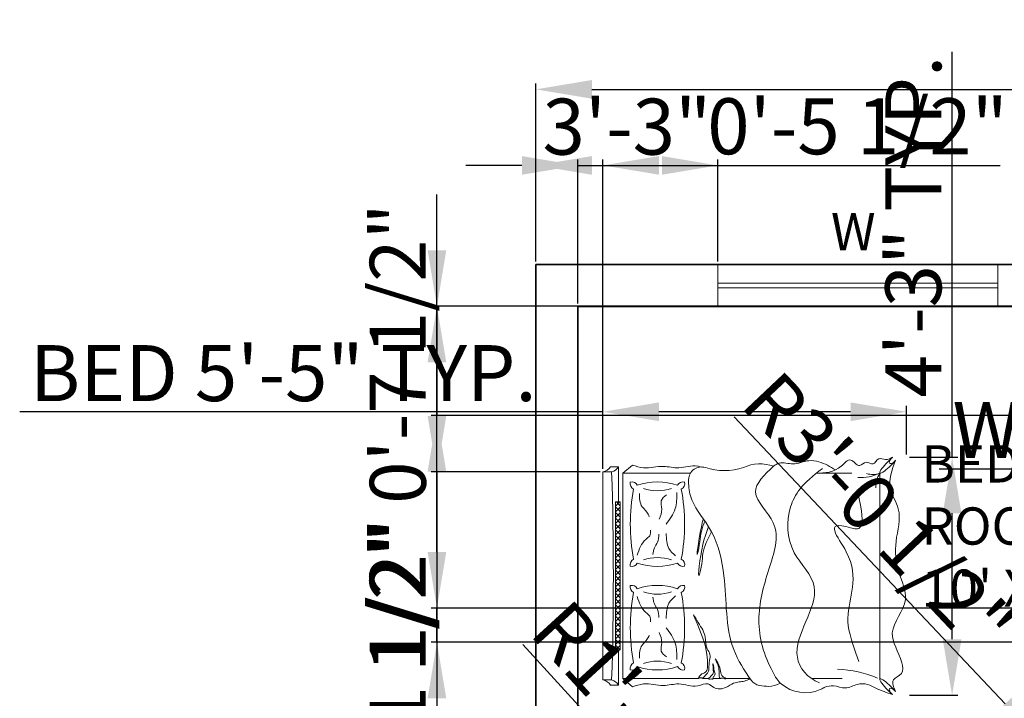
# Model space of a CAD drawing. Units: inches. Extents: x 2122 to 2726, y 1923 to 2370.
# Tile 3 of 6: x 2122 to 2333, y 2178 to 2324. Entities that reach past the tile are written whole.
import ezdxf

# ---------------------------------------------------------------- set-up
doc = ezdxf.new("R2010")
doc.units = ezdxf.units.IN
for name, color, linetype, lineweight in [('A-ANNO-DIMS', 2, 'Continuous', 18), ('A-ANNO-TEXT', 7, 'Continuous', 18), ('A-AREA-IDEN', 7, 'Continuous', 25), ('A-FURN', 8, 'Continuous', 18), ('A-GLAZ', 4, 'Continuous', 18), ('A-WALL', 7, 'Continuous', 35), ('www.cadblocksfree.com', 7, 'Continuous', 9)]:
    doc.layers.add(name, color=color, linetype=linetype, lineweight=lineweight)
doc.styles.get("Standard").update_dxf_attribs({"font": 'arial.ttf'})
doc.dimstyles.new('ISO-25', dxfattribs={"dimtxt": 12, "dimasz": 12, "dimexe": 1.25, "dimexo": 0.625, "dimtad": 1, "dimlunit": 3, "dimtxsty": 'Standard', "dimcen": 2.5, "dimadec": 0, "dimazin": 0, "dimtfac": 1, "dimtmove": 0, "dimatfit": 3, "dimfxl": 1, "dimarcsym": 0})

# ---------------------------------------------------------------- blocks, each defined once
blk = doc.blocks.new('bed')
at = {"layer": 'www.cadblocksfree.com', "ltscale": 0.2}
h = blk.add_hatch(dxfattribs=at)
h.set_pattern_fill('ANSI37,_O', color=256, scale=0.393701)
h.set_pattern_definition([(45, (2420.7222, -262.9689), (-0.8838835, 0.8838835), []), (135, (2420.7222, -262.9689), (-0.8838835, -0.8838835), [])])
h.paths.add_polyline_path([(3417.57, 1472.4), (3372.19, 1472.4), (3372.19, 1470.94), (3417.57, 1470.94)])
for p, q in [((3363, 1473.59), (3363, 1476.25)), ((3426.76, 1473.59), (3426.76, 1476.25)), ((3363.39, 1470.15), (3360.88, 1467.22)), ((3372.19, 1472.4), (3417.57, 1472.4)), ((3372.19, 1470.94), (3372.19, 1472.4)), ((3372.19, 1470.94), (3417.57, 1470.94)), ((3417.57, 1470.94), (3417.57, 1472.4)), ((3426.38, 1470.15), (3428.88, 1467.22)), ((3409.94, 1443.85), (3408.41, 1442.96)), ((3363.39, 1412.3), (3363.39, 1402.94)), ((3426.38, 1399.91), (3426.38, 1410.81)), ((3363.39, 1391.41), (3426.38, 1391.41))]:
    blk.add_line(p, q, dxfattribs=at)
for points in [[(3426.76, 1476.25), (3363, 1476.25)], [(3361.42, 1473.89), (3361.42, 1471.52), (3372.19, 1471.52)], [(3417.57, 1471.52), (3428.35, 1471.52), (3428.35, 1473.89)], [(3426.38, 1449.41), (3426.38, 1470.15), (3363.39, 1470.15), (3363.39, 1447.08)], [(3363.39, 1445.54), (3363.39, 1443.89)], [(3363.39, 1442.49), (3363.39, 1440.37)], [(3363.39, 1438.56), (3363.39, 1431.14)]]:
    blk.add_lwpolyline(points, dxfattribs=at)
for centre, radius, start, end in [((3359.33, 1477), 3.74, 303.8271, 348.4775), ((3430.43, 1477), 3.74, 191.5225, 236.1729), ((3359.84, 1474.37), 3.25, 298.9176, 345.9939), ((3394.88, 2431.36), 958.3, 268.09356, 271.90644), ((3429.92, 1474.37), 3.25, 194.0061, 241.0824), ((3367.9, 1467.4), 1.87, 165.5166, 244.2099), ((3366.56, 1466.05), 1.87, 25.7901, 104.4834), ((3379.01, 1409.19), 58.68, 79.4235, 100.5765), ((3391.47, 1466.05), 1.87, 75.5166, 154.2099), ((3390.12, 1467.4), 1.87, 295.7901, 14.4834), ((3399.64, 1467.4), 1.87, 165.5166, 244.2099), ((3398.3, 1466.05), 1.87, 25.7901, 104.4834), ((3410.75, 1409.19), 58.68, 79.4235, 100.5765), ((3423.21, 1466.05), 1.87, 75.5166, 154.2099), ((3421.86, 1467.4), 1.87, 295.7901, 14.4834), ((3385.29, 1459.55), 19.22, 161.2852, 198.7148), ((3355.42, 1459.55), 13.34, 341.1598, 18.8402), ((3402.61, 1459.55), 13.34, 161.1598, 198.8402), ((3372.74, 1459.55), 19.22, 341.2852, 18.7148), ((3417.03, 1459.55), 19.22, 161.2852, 198.7148), ((3387.15, 1459.55), 13.34, 341.1598, 18.8402), ((3434.35, 1459.55), 13.34, 161.1598, 198.8402), ((3404.48, 1459.55), 19.22, 341.2852, 18.7148), ((3367.9, 1451.7), 1.87, 115.7901, 194.4834), ((3366.56, 1453.04), 1.87, 255.5166, 334.2099), ((3379.01, 1509.91), 58.68, 259.4235, 280.5765), ((3391.47, 1453.04), 1.87, 205.7901, 284.4834), ((3390.12, 1451.7), 1.87, 345.5166, 64.2099), ((3399.64, 1451.7), 1.87, 115.7901, 194.4834), ((3398.3, 1453.04), 1.87, 255.5166, 334.2099), ((3410.75, 1509.91), 58.68, 259.4235, 280.5765), ((3423.21, 1453.04), 1.87, 205.7901, 284.4834), ((3421.86, 1451.7), 1.87, 345.5166, 64.2099), ((3424.34, 1446.05), 3.94, 342.0511, 87.9851), ((3445.78, 1439.1), 18.6, 162.0511, 198.5657), ((3365.21, 1427.6), 3.94, 125.4209, 169.6982), ((3416.57, 1428.08), 12.65, 341.0268, 23.7782), ((3370.55, 1414.19), 11.47, 139.4648, 203.3712), ((3367.28, 1412.87), 7.94, 204.0179, 212.619), ((3331.91, 1405.56), 34.38, 336.8495, 357.9003), ((3438.82, 1397.31), 13.77, 176.7525, 205.373), ((3432.14, 1393.64), 6.17, 162.6475, 201.1361), ((3422.11, 1384.8), 7.8, 58.0013, 91.6551)]:
    blk.add_arc(centre, radius, start, end, dxfattribs=at)
at = {"layer": 'www.cadblocksfree.com', "ltscale": 0.2, "extrusion": (0, 0, -1)}
for centre, major_axis, ratio, start_param, end_param in [((3360.34, 1388.37), (3.04, 3.04), 0.168252, 4.250342, 8.316029), ((3359.29, 1387.32), (1.05, 1.05), 0.453532, 4.422107, 8.144264)]:
    blk.add_ellipse(centre, major_axis=major_axis, ratio=ratio, start_param=start_param, end_param=end_param, dxfattribs=at)
at = {"layer": 'www.cadblocksfree.com', "ltscale": 0.2}
for centre, major_axis, ratio, start_param, end_param in [((3429.42, 1388.37), (-3.04, 3.04), 0.168252, 4.250342, 8.316029), ((3430.48, 1387.32), (-1.05, 1.05), 0.453532, 4.422107, 8.144264)]:
    blk.add_ellipse(centre, major_axis=major_axis, ratio=ratio, start_param=start_param, end_param=end_param, dxfattribs=at)
for points, knots in [([(3360.88, 1467.22), (3361.27, 1466.08), (3362.33, 1462.98), (3360.73, 1458.15), (3362.39, 1452.62), (3360.35, 1448.14), (3362.43, 1444.24), (3360.04, 1441.93), (3360.26, 1438.68), (3362.05, 1436.55), (3362.42, 1434.52), (3362.57, 1432.76), (3363.1, 1431.71), (3363.39, 1431.14)], [0, 0, 0, 0, 3.550403, 9.643115, 14.356056, 20.206026, 23.427697, 25.46537, 29.172767, 31.884544, 33.668442, 35.237641, 37.145618, 37.145618, 37.145618, 37.145618]), ([(3428.88, 1467.22), (3428.49, 1466.08), (3427.44, 1462.98), (3429.04, 1458.15), (3427.38, 1452.62), (3429.08, 1448.87), (3428.37, 1446.52), (3428.27, 1446.19)], [0, 0, 0, 0, 0.0901802, 0.2449351, 0.3646438, 0.5132331, 0.5378548, 0.5378548, 0.5378548, 0.5378548]), ([(3369.63, 1465.08), (3371.1, 1465.04), (3373.63, 1464.97), (3375.26, 1462.52), (3376.48, 1462.17), (3376.75, 1462.09)], [0, 0, 0, 0, 4.163459, 7.093919, 7.934624, 7.934624, 7.934624, 7.934624]), ([(3388.54, 1465.74), (3386.72, 1465.16), (3384.36, 1464.41), (3382.68, 1461.63), (3381.45, 1461.64), (3380.81, 1461.64)], [0, 0, 0, 0, 5.530688, 7.154877, 8.940839, 8.940839, 8.940839, 8.940839]), ([(3401.22, 1465.74), (3403.05, 1465.16), (3405.41, 1464.41), (3407.09, 1461.63), (3408.31, 1461.64), (3408.95, 1461.64)], [0, 0, 0, 0, 5.530688, 7.154877, 8.940839, 8.940839, 8.940839, 8.940839]), ([(3420.14, 1465.08), (3418.66, 1465.04), (3416.14, 1464.97), (3414.5, 1462.52), (3413.28, 1462.17), (3413.01, 1462.09)], [0, 0, 0, 0, 4.163459, 7.093919, 7.934624, 7.934624, 7.934624, 7.934624]), ([(3388.36, 1460.93), (3387.64, 1460.85), (3386.25, 1460.69), (3384.48, 1459.22), (3382.96, 1459.13), (3382.11, 1459.07)], [0, 0, 0, 0, 2.127543, 4.10272, 6.58647, 6.58647, 6.58647, 6.58647]), ([(3401.41, 1460.93), (3402.13, 1460.85), (3403.51, 1460.69), (3405.28, 1459.22), (3406.81, 1459.13), (3407.65, 1459.07)], [0, 0, 0, 0, 2.127543, 4.10272, 6.58647, 6.58647, 6.58647, 6.58647]), ([(3370.05, 1456.77), (3370.59, 1457.46), (3371.71, 1458.88), (3374.68, 1457.89), (3376.51, 1458.59), (3377.52, 1458.99)], [0, 0, 0, 0, 2.388143, 4.935423, 8.166198, 8.166198, 8.166198, 8.166198]), ([(3419.72, 1456.77), (3419.17, 1457.46), (3418.05, 1458.88), (3415.08, 1457.89), (3413.26, 1458.59), (3412.24, 1458.99)], [0, 0, 0, 0, 2.388143, 4.935423, 8.166198, 8.166198, 8.166198, 8.166198]), ([(3369.29, 1453.58), (3371, 1453.6), (3374.59, 1453.64), (3377.5, 1455.76), (3379.02, 1456.87)], [0, 0, 0, 0, 5.002087, 10.507046, 10.507046, 10.507046, 10.507046]), ([(3388.77, 1454), (3388.07, 1454.76), (3386.27, 1456.73), (3383.54, 1456.81), (3381.88, 1456.86)], [0, 0, 0, 0, 3.013696, 7.735839, 7.735839, 7.735839, 7.735839]), ([(3401, 1454), (3401.7, 1454.76), (3403.5, 1456.73), (3406.22, 1456.81), (3407.88, 1456.86)], [0, 0, 0, 0, 3.013696, 7.735839, 7.735839, 7.735839, 7.735839]), ([(3420.48, 1453.58), (3418.77, 1453.6), (3415.18, 1453.64), (3412.27, 1455.76), (3410.74, 1456.87)], [0, 0, 0, 0, 5.002087, 10.507046, 10.507046, 10.507046, 10.507046]), ([(3367.27, 1444.2), (3369.57, 1444.23), (3373.92, 1444.28), (3385.47, 1449.8), (3379.56, 1446.49), (3376.81, 1444.48), (3372.95, 1444.92), (3370.93, 1443.14), (3368.77, 1443.7), (3367.36, 1443.75), (3366.55, 1443.78)], [0, 0, 0, 0, 8.61026, 16.221274, 18.843057, 23.804898, 27.440828, 29.356102, 31.203478, 33.650687, 33.650687, 33.650687, 33.650687]), ([(3409.94, 1443.85), (3413.12, 1445.84), (3417.43, 1449.66), (3422.72, 1450.04), (3424.48, 1449.98)], [1.3582378, 1.3582378, 1.3582378, 1.3582378, 1.6381418, 1.7706953, 1.7706953, 1.7706953, 1.7706953]), ([(3363.39, 1447.08), (3363.43, 1446.99), (3363.53, 1446.78), (3363.73, 1446.46), (3363.51, 1446.15), (3363.66, 1445.9), (3363.56, 1445.67), (3363.44, 1445.58), (3363.39, 1445.54)], [0, 0, 0, 0, 0.293454, 0.701471, 1.003873, 1.254893, 1.47342, 1.69185, 1.69185, 1.69185, 1.69185]), ([(3363.39, 1447.08), (3363.99, 1446.78), (3365.08, 1446.12), (3365.12, 1444.37), (3367.13, 1444.19), (3367.27, 1444.2)], [0.0122268, 0.0122268, 0.0122268, 0.0122268, 0.0594721, 0.1062177, 0.134458, 0.134458, 0.134458, 0.134458]), ([(3409.94, 1443.85), (3408.47, 1444.45), (3404.44, 1446.04), (3391.4, 1447.6), (3398.64, 1445.77), (3402.97, 1445.76), (3406.22, 1444.09), (3408.41, 1442.96)], [0.0056315, 0.0056315, 0.0056315, 0.0056315, 0.1489731, 0.3882761, 0.4793617, 0.5593494, 0.7397317, 0.7397317, 0.7397317, 0.7397317]), ([(3412.4, 1445.5), (3411.61, 1445.7), (3406.24, 1446.93), (3398.17, 1447.93), (3405.4, 1446.46), (3408.57, 1446.19), (3410.63, 1445.46), (3411.68, 1445)], [0.1043639, 0.1043639, 0.1043639, 0.1043639, 0.1489731, 0.3882761, 0.4793617, 0.5593494, 0.6446217, 0.6446217, 0.6446217, 0.6446217]), ([(3362.93, 1430.81), (3365.94, 1432.96), (3375.45, 1438.99), (3392.12, 1438.03), (3404.25, 1440.73), (3408.41, 1442.96)], [0.102872, 0.102872, 0.102872, 0.102872, 0.37972, 0.957702, 1.313793, 1.313793, 1.313793, 1.313793]), ([(3363.39, 1443.89), (3363.33, 1443.81), (3363.17, 1443.56), (3363.35, 1443.12), (3363.23, 1442.79), (3363.23, 1442.53), (3363.34, 1442.51), (3363.39, 1442.49)], [0, 0, 0, 0, 0.27176, 0.887321, 1.189132, 1.388142, 1.515331, 1.515331, 1.515331, 1.515331]), ([(3366.55, 1443.78), (3366.17, 1443.78), (3365.17, 1443.9), (3364.4, 1444.96), (3363.63, 1445.46), (3363.39, 1445.54)], [0.15648839, 0.15648839, 0.15648839, 0.15648839, 0.18439755, 0.23137648, 0.25059846, 0.25059846, 0.25059846, 0.25059846]), ([(3363.39, 1443.89), (3363.63, 1443.61), (3364.67, 1442.73), (3364.89, 1442.15), (3369.07, 1442.74), (3366.77, 1442.24), (3365.83, 1442.3), (3364.61, 1441.55), (3363.96, 1442.54), (3363.54, 1442.52), (3363.39, 1442.49)], [0.0595743, 0.0595743, 0.0595743, 0.0595743, 0.0807529, 0.1037415, 0.1697201, 0.1760361, 0.2071372, 0.2404744, 0.2623409, 0.2736605, 0.2736605, 0.2736605, 0.2736605]), ([(3363.39, 1440.37), (3363.44, 1440.27), (3363.57, 1440.06), (3363.61, 1439.68), (3363.53, 1439.31), (3363.41, 1439), (3363.33, 1438.75), (3363.37, 1438.61), (3363.39, 1438.56)], [0, 0, 0, 0, 0.329977, 0.725302, 1.129072, 1.442831, 1.734218, 1.878348, 1.878348, 1.878348, 1.878348]), ([(3363.39, 1440.37), (3363.63, 1440.51), (3364.53, 1440.9), (3366.48, 1440.25), (3370.2, 1442.29), (3367.73, 1440.64), (3365.42, 1440.07), (3364.04, 1439.91), (3363.8, 1438.94), (3363.48, 1438.64), (3363.39, 1438.56)], [0.013856, 0.013856, 0.013856, 0.013856, 0.0348738, 0.0888667, 0.1078792, 0.1267378, 0.158714, 0.1937575, 0.2174868, 0.2267221, 0.2267221, 0.2267221, 0.2267221]), ([(3361.34, 1428.31), (3361.33, 1428.3), (3361.16, 1427.34), (3360.78, 1425.17), (3361.47, 1423.14), (3362.01, 1421.85)], [0.3128349, 0.3128349, 0.3128349, 0.3128349, 0.313751, 0.386958, 0.4759027, 0.4759027, 0.4759027, 0.4759027]), ([(3365.51, 1424.21), (3370.52, 1427), (3381.15, 1429.83), (3396.21, 1425.87), (3410.54, 1420.65), (3420.27, 1432.69), (3425.88, 1426.77), (3428.53, 1423.97)], [0.099185, 0.099185, 0.099185, 0.099185, 0.523647, 0.927087, 1.289918, 1.564439, 1.810555, 1.810555, 1.810555, 1.810555]), ([(3428.53, 1423.97), (3428.91, 1423.4), (3430.1, 1421.61), (3428.49, 1417.66), (3430.59, 1413.79), (3429.8, 1409.12), (3428.4, 1406.56), (3427.36, 1404.97)], [0, 0, 0, 0, 0.050513, 0.157399, 0.2842023, 0.3628173, 0.5066917, 0.5066917, 0.5066917, 0.5066917]), ([(3362.06, 1409.87), (3363.64, 1413.65), (3372.98, 1421.34), (3389.68, 1406.04), (3402.4, 1419.98), (3416.04, 1420.17), (3423.23, 1415.23), (3427.83, 1408.9)], [0.029901, 0.029901, 0.029901, 0.029901, 0.276967, 0.797115, 1.093669, 1.464666, 1.788489, 1.788489, 1.788489, 1.788489]), ([(3431.24, 1387.47), (3430.88, 1388.17), (3430.2, 1389.5), (3431.48, 1391.99), (3428.29, 1393.19), (3430.5, 1395.69), (3427.56, 1397.87), (3431.84, 1400.39), (3426.54, 1404.33), (3426.44, 1408.15), (3426.38, 1410.81)], [0, 0, 0, 0, 2.267059, 4.324559, 6.685584, 8.878641, 11.121502, 14.300359, 17.755284, 25.682856, 25.682856, 25.682856, 25.682856]), ([(3358.53, 1387.47), (3359.1, 1389.21), (3359.96, 1391.82), (3361.92, 1395.15), (3361.9, 1398.55), (3359.88, 1401.84), (3361.56, 1405.21), (3361.03, 1407.51), (3360.64, 1408.47), (3360.59, 1408.59)], [0, 0, 0, 0, 0.138875, 0.2092702, 0.2901949, 0.3858479, 0.4804923, 0.5489252, 0.5590752, 0.5590752, 0.5590752, 0.5590752]), ([(3368.63, 1397.84), (3375.98, 1400.49), (3385.35, 1402.76), (3397.53, 1395.27), (3413.59, 1410.38), (3407.81, 1395.02), (3420.76, 1398.2)], [0.029901, 0.029901, 0.029901, 0.029901, 0.276967, 0.797115, 1.093669, 1.16836, 1.16836, 1.16836, 1.16836]), ([(3430.32, 1386.56), (3427.33, 1387.65), (3422.15, 1389.55), (3414.53, 1384.14), (3405.61, 1387.05), (3396.29, 1386.31), (3386.84, 1381.28), (3377.74, 1390.27), (3370.78, 1384.8), (3364.63, 1383.97), (3363.28, 1388.27), (3360.78, 1387.15), (3359.45, 1386.56)], [0, 0, 0, 0, 8.93042, 15.449194, 25.485629, 34.878505, 43.598887, 54.554403, 64.16647, 67.461673, 70.610457, 74.213583, 74.213583, 74.213583, 74.213583])]:
    blk.add_open_spline(points, degree=3, knots=knots, dxfattribs=at)
for points in [[(3361.23, 1424.04), (3361.24, 1424.04), (3361.24, 1424.04), (3361.24, 1424.04)], [(3361.84, 1421.64), (3362.35, 1422.25), (3362.87, 1422.86), (3365.51, 1424.21)]]:
    blk.add_open_spline(points, degree=3, dxfattribs=at)
blk = doc.blocks.new('*D10')
at = {"layer": 'A-ANNO-DIMS', "color": 0, "lineweight": -2, "transparency": 16777216}
for p, q in [((2232.51, 2271.86), (2232.51, 2309.99)), ((2244.51, 2308.74), (2588.01, 2308.74)), ((2600.01, 2271.86), (2600.01, 2309.99))]:
    blk.add_line(p, q, dxfattribs=at)
at = {"layer": 'A-ANNO-DIMS', "color": 0, "transparency": 16777216}
for points in [[(2244.51, 2310.74), (2244.51, 2306.74), (2232.51, 2308.74)], [(2588.01, 2310.74), (2588.01, 2306.74), (2600.01, 2308.74)]]:
    blk.add_solid(points, dxfattribs=at)
at = {"layer": 'Defpoints', "color": 0, "transparency": 16777216}
for p in [(2600.01, 2308.74), (2232.51, 2271.24), (2600.01, 2271.24)]:
    blk.add_point(p, dxfattribs=at)
at = {"layer": 'A-ANNO-DIMS', "color": 0, "transparency": 16777216, "insert": (2416.26, 2315.49), "char_height": 12, "attachment_point": 5}
blk.add_mtext("31'", dxfattribs=at)
blk = doc.blocks.new('WIN-60IN')
for p, q in [((0, 0), (0, 9)), ((60, 0), (60, 9)), ((0, 5), (60, 5)), ((0, 4), (60, 4))]:
    blk.add_line(p, q)
blk = doc.blocks.new('*D22')
at = {"layer": 'A-ANNO-DIMS', "color": 0, "lineweight": -2, "transparency": 16777216}
for p, q in [((2330.01, 2144.86), (2330.01, 2150.89)), ((2366.01, 2144.86), (2366.01, 2150.89)), ((2330.01, 2149.64), (2142.68, 2149.64)), ((2354.01, 2149.64), (2342.01, 2149.64))]:
    blk.add_line(p, q, dxfattribs=at)
at = {"layer": 'A-ANNO-DIMS', "color": 0, "transparency": 16777216}
for points in [[(2342.01, 2151.64), (2342.01, 2147.64), (2330.01, 2149.64)], [(2354.01, 2151.64), (2354.01, 2147.64), (2366.01, 2149.64)]]:
    blk.add_solid(points, dxfattribs=at)
at = {"layer": 'Defpoints', "color": 0, "transparency": 16777216}
for p in [(2330.01, 2149.64), (2330.01, 2144.24), (2366.01, 2144.24)]:
    blk.add_point(p, dxfattribs=at)
at = {"layer": 'A-ANNO-DIMS', "color": 0, "transparency": 16777216, "insert": (2230.34, 2156.47), "char_height": 12, "attachment_point": 5}
blk.add_mtext('DOOR LEAF 3\'-0" TYP.', dxfattribs=at)
blk = doc.blocks.new('*D26')
at = {"layer": 'A-ANNO-DIMS', "color": 0, "lineweight": -2, "transparency": 16777216}
for p, q in [((2246.89, 2230.5), (2246.89, 2240.89)), ((2311.95, 2230.5), (2311.95, 2240.89)), ((2246.89, 2239.64), (2121.9, 2239.64)), ((2299.95, 2239.64), (2258.89, 2239.64))]:
    blk.add_line(p, q, dxfattribs=at)
at = {"layer": 'A-ANNO-DIMS', "color": 0, "transparency": 16777216}
for points in [[(2258.89, 2241.64), (2258.89, 2237.64), (2246.89, 2239.64)], [(2299.95, 2241.64), (2299.95, 2237.64), (2311.95, 2239.64)]]:
    blk.add_solid(points, dxfattribs=at)
at = {"layer": 'Defpoints', "color": 0, "transparency": 16777216}
for p in [(2246.89, 2239.64), (2246.89, 2229.88), (2311.95, 2229.88)]:
    blk.add_point(p, dxfattribs=at)
at = {"layer": 'A-ANNO-DIMS', "color": 0, "transparency": 16777216, "insert": (2178.39, 2246.37), "char_height": 12, "attachment_point": 5}
blk.add_mtext('BED 5\'-5" TYP.', dxfattribs=at)
blk = doc.blocks.new('*D27')
at = {"layer": 'A-ANNO-DIMS', "color": 0, "lineweight": -2, "transparency": 16777216}
for p, q in [((2321.71, 2229.88), (2321.71, 2316.76)), ((2312.58, 2229.88), (2322.96, 2229.88)), ((2321.71, 2190.88), (2321.71, 2217.88)), ((2312.58, 2178.88), (2322.96, 2178.88))]:
    blk.add_line(p, q, dxfattribs=at)
at = {"layer": 'A-ANNO-DIMS', "color": 0, "transparency": 16777216}
for points in [[(2319.71, 2217.88), (2323.71, 2217.88), (2321.71, 2229.88)], [(2319.71, 2190.88), (2323.71, 2190.88), (2321.71, 2178.88)]]:
    blk.add_solid(points, dxfattribs=at)
at = {"layer": 'Defpoints', "color": 0, "transparency": 16777216}
for p in [(2311.95, 2229.88), (2321.71, 2229.88), (2311.95, 2178.88)]:
    blk.add_point(p, dxfattribs=at)
at = {"layer": 'A-ANNO-DIMS', "color": 0, "transparency": 16777216, "insert": (2314.95, 2279.32), "char_height": 12, "attachment_point": 5, "rotation": 90}
blk.add_mtext('4\'-3" TYP.', dxfattribs=at)
blk = doc.blocks.new('*D28')
at = {"layer": 'A-ANNO-DIMS', "color": 0, "lineweight": -2, "transparency": 16777216}
for p, q in [((2450.4, 2228.51), (2450.4, 2226.12)), ((2462.17, 2228.51), (2462.17, 2226.12)), ((2438.4, 2227.37), (2318.92, 2227.37)), ((2462.17, 2227.37), (2450.4, 2227.37)), ((2474.17, 2227.37), (2486.17, 2227.37))]:
    blk.add_line(p, q, dxfattribs=at)
at = {"layer": 'A-ANNO-DIMS', "color": 0, "transparency": 16777216}
for points in [[(2438.4, 2229.37), (2438.4, 2225.37), (2450.4, 2227.37)], [(2474.17, 2229.37), (2474.17, 2225.37), (2462.17, 2227.37)]]:
    blk.add_solid(points, dxfattribs=at)
at = {"layer": 'Defpoints', "color": 0, "transparency": 16777216}
for p in [(2450.4, 2229.14), (2462.17, 2229.14), (2450.4, 2227.37)]:
    blk.add_point(p, dxfattribs=at)
at = {"layer": 'A-ANNO-DIMS', "color": 0, "transparency": 16777216, "insert": (2372.66, 2234.2), "char_height": 12, "attachment_point": 5}
blk.add_mtext('WC 1\'-0" TYP.', dxfattribs=at)
blk = doc.blocks.new('*D41')
at = {"layer": 'A-ANNO-DIMS', "color": 0, "lineweight": -2, "transparency": 16777216}
for p, q in [((2232.51, 2271.86), (2232.51, 2293.69)), ((2271.51, 2271.86), (2271.51, 2293.69)), ((2244.51, 2292.44), (2259.51, 2292.44))]:
    blk.add_line(p, q, dxfattribs=at)
at = {"layer": 'A-ANNO-DIMS', "color": 0, "transparency": 16777216}
for points in [[(2244.51, 2294.44), (2244.51, 2290.44), (2232.51, 2292.44)], [(2259.51, 2294.44), (2259.51, 2290.44), (2271.51, 2292.44)]]:
    blk.add_solid(points, dxfattribs=at)
at = {"layer": 'Defpoints', "color": 0, "transparency": 16777216}
for p in [(2271.51, 2292.44), (2232.51, 2271.24), (2271.51, 2271.24)]:
    blk.add_point(p, dxfattribs=at)
at = {"layer": 'A-ANNO-DIMS', "color": 0, "transparency": 16777216, "insert": (2252.01, 2299.19), "char_height": 12, "attachment_point": 5}
blk.add_mtext('3\'-3"', dxfattribs=at)
blk = doc.blocks.new('*D51')
at = {"layer": 'A-ANNO-DIMS', "color": 0, "lineweight": -2, "transparency": 16777216}
for p, q in [((2211.31, 2209.57), (2211.31, 2282.68)), ((2465.88, 2197.57), (2210.06, 2197.57)), ((2211.31, 2190.24), (2211.31, 2197.57)), ((2465.88, 2190.24), (2210.06, 2190.24)), ((2211.31, 2178.24), (2211.31, 2166.24))]:
    blk.add_line(p, q, dxfattribs=at)
at = {"layer": 'A-ANNO-DIMS', "color": 0, "transparency": 16777216}
for points in [[(2209.31, 2209.57), (2213.31, 2209.57), (2211.31, 2197.57)], [(2209.31, 2178.24), (2213.31, 2178.24), (2211.31, 2190.24)]]:
    blk.add_solid(points, dxfattribs=at)
at = {"layer": 'Defpoints', "color": 0, "transparency": 16777216}
for p in [(2211.31, 2197.57), (2466.51, 2197.57), (2466.51, 2190.24)]:
    blk.add_point(p, dxfattribs=at)
at = {"layer": 'A-ANNO-DIMS', "color": 0, "transparency": 16777216, "insert": (2204.48, 2252.12), "char_height": 12, "attachment_point": 5, "rotation": 90}
blk.add_mtext('0\'-7 1/2"', dxfattribs=at)
blk = doc.blocks.new('*D60')
at = {"layer": 'A-ANNO-DIMS', "color": 0, "lineweight": -2, "transparency": 16777216}
for p, q in [((2241.51, 2262.86), (2241.51, 2293.69)), ((2246.89, 2227.38), (2246.89, 2293.69)), ((2229.51, 2292.44), (2217.51, 2292.44)), ((2241.51, 2292.44), (2246.89, 2292.44)), ((2258.89, 2292.44), (2332, 2292.44))]:
    blk.add_line(p, q, dxfattribs=at)
at = {"layer": 'A-ANNO-DIMS', "color": 0, "transparency": 16777216}
for points in [[(2229.51, 2294.44), (2229.51, 2290.44), (2241.51, 2292.44)], [(2258.89, 2294.44), (2258.89, 2290.44), (2246.89, 2292.44)]]:
    blk.add_solid(points, dxfattribs=at)
at = {"layer": 'Defpoints', "color": 0, "transparency": 16777216}
for p in [(2246.89, 2292.44), (2241.51, 2262.24), (2246.89, 2226.75)]:
    blk.add_point(p, dxfattribs=at)
at = {"layer": 'A-ANNO-DIMS', "color": 0, "transparency": 16777216, "insert": (2301.44, 2299.27), "char_height": 12, "attachment_point": 5}
blk.add_mtext('0\'-5 1/2"', dxfattribs=at)
blk = doc.blocks.new('*D61')
at = {"layer": 'A-ANNO-DIMS', "color": 0, "lineweight": -2, "transparency": 16777216}
for p, q in [((2240.88, 2262.24), (2210.06, 2262.24)), ((2211.31, 2250.24), (2211.31, 2238.75)), ((2246.26, 2226.75), (2210.06, 2226.75)), ((2211.31, 2226.75), (2211.31, 2144.11))]:
    blk.add_line(p, q, dxfattribs=at)
at = {"layer": 'A-ANNO-DIMS', "color": 0, "transparency": 16777216}
for points in [[(2209.31, 2250.24), (2213.31, 2250.24), (2211.31, 2262.24)], [(2209.31, 2238.75), (2213.31, 2238.75), (2211.31, 2226.75)]]:
    blk.add_solid(points, dxfattribs=at)
at = {"layer": 'Defpoints', "color": 0, "transparency": 16777216}
for p in [(2241.51, 2262.24), (2211.31, 2226.75), (2246.89, 2226.75)]:
    blk.add_point(p, dxfattribs=at)
at = {"layer": 'A-ANNO-DIMS', "color": 0, "transparency": 16777216, "insert": (2204.48, 2179.43), "char_height": 12, "attachment_point": 5, "rotation": 90}
blk.add_mtext('2\'-11 1/2"', dxfattribs=at)
blk = doc.blocks.new('*D65')
at = {"layer": 'A-ANNO-DIMS', "color": 0, "lineweight": -2, "transparency": 16777216}
for p, q in [((2211.31, 2274.24), (2211.31, 2286.24)), ((2413.38, 2262.24), (2210.06, 2262.24)), ((2211.31, 2262.24), (2211.31, 2238.81)), ((2409.54, 2238.81), (2210.06, 2238.81)), ((2211.31, 2226.81), (2211.31, 2145.5))]:
    blk.add_line(p, q, dxfattribs=at)
at = {"layer": 'A-ANNO-DIMS', "color": 0, "transparency": 16777216}
for points in [[(2209.31, 2274.24), (2213.31, 2274.24), (2211.31, 2262.24)], [(2209.31, 2226.81), (2213.31, 2226.81), (2211.31, 2238.81)]]:
    blk.add_solid(points, dxfattribs=at)
at = {"layer": 'Defpoints', "color": 0, "transparency": 16777216}
for p in [(2414.01, 2262.24), (2211.31, 2238.81), (2410.17, 2238.81)]:
    blk.add_point(p, dxfattribs=at)
at = {"layer": 'A-ANNO-DIMS', "color": 0, "transparency": 16777216, "insert": (2204.48, 2180.16), "char_height": 12, "attachment_point": 5, "rotation": 90}
blk.add_mtext('1\'-11 1/2"', dxfattribs=at)
blk = doc.blocks.new('*D70')
at = {"layer": 'A-ANNO-DIMS', "color": 0, "lineweight": -2, "transparency": 16777216}
for p, q in [((2274.99, 2238.55), (2333.07, 2177.05)), ((2366.24, 2141.93), (2341.31, 2168.33))]:
    blk.add_line(p, q, dxfattribs=at)
at = {"layer": 'A-ANNO-DIMS', "color": 0, "transparency": 16777216}
blk.add_solid([(2334.53, 2178.42), (2331.62, 2175.68), (2341.31, 2168.33)], dxfattribs=at)
at = {"layer": 'Defpoints', "color": 0, "transparency": 16777216}
for p in [(2341.31, 2168.33), (2366.24, 2141.93)]:
    blk.add_point(p, dxfattribs=at)
at = {"layer": 'A-ANNO-DIMS', "color": 0, "transparency": 16777216, "insert": (2304.88, 2216.85), "char_height": 12, "attachment_point": 5, "rotation": 313.3629}
blk.add_mtext('R3\'-0 1/2"', dxfattribs=at)
blk = doc.blocks.new('*D73')
at = {"layer": 'A-ANNO-DIMS', "color": 0, "lineweight": -2, "transparency": 16777216}
for p, q in [((2229.71, 2189.76), (2293.17, 2120.53)), ((2316.45, 2095.14), (2301.28, 2111.68))]:
    blk.add_line(p, q, dxfattribs=at)
at = {"layer": 'A-ANNO-DIMS', "color": 0, "transparency": 16777216}
blk.add_solid([(2294.65, 2121.88), (2291.7, 2119.18), (2301.28, 2111.68)], dxfattribs=at)
at = {"layer": 'Defpoints', "color": 0, "transparency": 16777216}
for p in [(2301.28, 2111.68), (2316.45, 2095.14)]:
    blk.add_point(p, dxfattribs=at)
at = {"layer": 'A-ANNO-DIMS', "color": 0, "transparency": 16777216, "insert": (2262.42, 2164.19), "char_height": 12, "attachment_point": 5, "rotation": 312.5099}
blk.add_mtext('R1\'-10 1/2"', dxfattribs=at)

msp = doc.modelspace()

# ---------------------------------------------------------------- linework, layer by layer
at = {"layer": 'A-WALL'}
for p, q in [((2232.508, 2271.236), (2600.008, 2271.236)), ((2232.508, 2271.236), (2232.508, 2142.236)), ((2241.508, 2262.236), (2361.508, 2262.236)), ((2241.508, 2262.236), (2241.508, 2142.236))]:
    msp.add_line(p, q, dxfattribs=at)

# ---------------------------------------------------------------- block references
at = {"layer": 'A-FURN', "xscale": 0.6990837586902172, "yscale": 0.6990837586902172, "zscale": 0.6990837586902172, "rotation": 89.99999999999999}
msp.add_blockref('bed', (3278.907, -168.843), dxfattribs=at)
at = {"layer": 'A-GLAZ'}
msp.add_blockref('WIN-60IN', (2271.508, 2262.236), dxfattribs=at)

# ---------------------------------------------------------------- texts
at = {"layer": 'A-ANNO-TEXT', "insert": (2295.748, 2282.226), "char_height": 7.99, "attachment_point": 1}
msp.add_mtext_dynamic_manual_height_columns('W', width=65.06795, gutter_width=39.949, heights=[0], dxfattribs=at)
at = {"layer": 'A-AREA-IDEN', "insert": (2315.153, 2232.468), "char_height": 7.9897, "attachment_point": 1}
msp.add_mtext_dynamic_manual_height_columns("BED\\PROOM \\P10' X 10'", width=65.06795, gutter_width=39.949, heights=[0], dxfattribs=at)

# ---------------------------------------------------------------- dimensions: what is measured, and where the dimension line sits
at = {"layer": 'A-ANNO-DIMS'}
dim = msp.add_linear_dim(base=(2600.008, 2308.735), p1=(2232.508, 2271.236), p2=(2600.008, 2271.236), text="31'", dimstyle='ISO-25', override={"dimclrd": 0, "dimclre": 0, "dimclrt": 0}, dxfattribs=at)
dim.commit()
dim.dimension.update_dxf_attribs({"geometry": '*D10', "text_midpoint": (2416.258, 2315.491)})
for base, p1, p2, picture, middle in [((2246.886, 2292.436), (2241.508, 2262.236), (2246.886, 2226.751), '*D60', (2301.441, 2299.266)), ((2271.508, 2292.436), (2232.508, 2271.236), (2271.508, 2271.236), '*D41', (2252.008, 2299.192))]:
    dim = msp.add_linear_dim(base=base, p1=p1, p2=p2, dimstyle='ISO-25', override={"dimdec": 1, "dimlfac": 1, "dimrnd": 0, "dimzin": 1, "dimdsep": 46, "dimlunit": 4, "dimfrac": 2}, dxfattribs=at)
    dim.commit()
    dim.dimension.update_dxf_attribs({"geometry": picture, "text_midpoint": middle})
for base, p1, p2, angle, text, picture, middle in [((2321.71, 2229.878), (2311.95, 2178.882), (2311.95, 2229.878), 90, '<> TYP.', '*D27', (2314.954, 2279.318)), ((2246.886, 2239.638), (2311.95, 2229.878), (2246.886, 2229.878), 180, 'BED <> TYP.', '*D26', (2178.39, 2246.365)), ((2450.397, 2227.374), (2462.172, 2229.14), (2450.397, 2229.14), 180, 'WC <> TYP.', '*D28', (2372.66, 2234.203)), ((2330.008, 2149.636), (2366.008, 2144.236), (2330.008, 2144.236), 180, 'DOOR LEAF <> TYP.', '*D22', (2230.342, 2156.474))]:
    dim = msp.add_linear_dim(base=base, p1=p1, p2=p2, angle=angle, text=text, dimstyle='ISO-25', override={"dimdec": 1, "dimlfac": 1, "dimrnd": 0, "dimzin": 1, "dimdsep": 46, "dimlunit": 4, "dimfrac": 2}, dxfattribs=at)
    dim.commit()
    dim.dimension.update_dxf_attribs({"geometry": picture, "text_midpoint": middle})
for base, p1, p2, picture, middle in [((2211.308, 2238.809), (2414.008, 2262.236), (2410.167, 2238.809), '*D65', (2204.478, 2180.156)), ((2211.308, 2197.569), (2466.508, 2190.236), (2466.508, 2197.569), '*D51', (2204.478, 2252.124)), ((2211.308, 2226.751), (2241.508, 2262.236), (2246.886, 2226.751), '*D61', (2204.478, 2179.432))]:
    dim = msp.add_linear_dim(base=base, p1=p1, p2=p2, angle=90, dimstyle='ISO-25', override={"dimdec": 1, "dimlfac": 1, "dimrnd": 0, "dimzin": 1, "dimdsep": 46, "dimlunit": 4, "dimfrac": 2}, dxfattribs=at)
    dim.commit()
    dim.dimension.update_dxf_attribs({"geometry": picture, "text_midpoint": middle})
for center, mpoint, picture, middle in [((2366.243, 2141.928), (2341.313, 2168.325), '*D70', (2304.88, 2216.855)), ((2316.451, 2095.138), (2301.283, 2111.685), '*D73', (2262.424, 2164.185))]:
    dim = msp.add_radius_dim(center=center, mpoint=mpoint, dimstyle='ISO-25', override={"dimdec": 1, "dimlfac": 1, "dimrnd": 0, "dimzin": 1, "dimdsep": 46, "dimlunit": 4, "dimfrac": 2}, dxfattribs=at)
    dim.commit()
    dim.dimension.update_dxf_attribs({"geometry": picture, "text_midpoint": middle})

doc.saveas('drawing.dxf')
